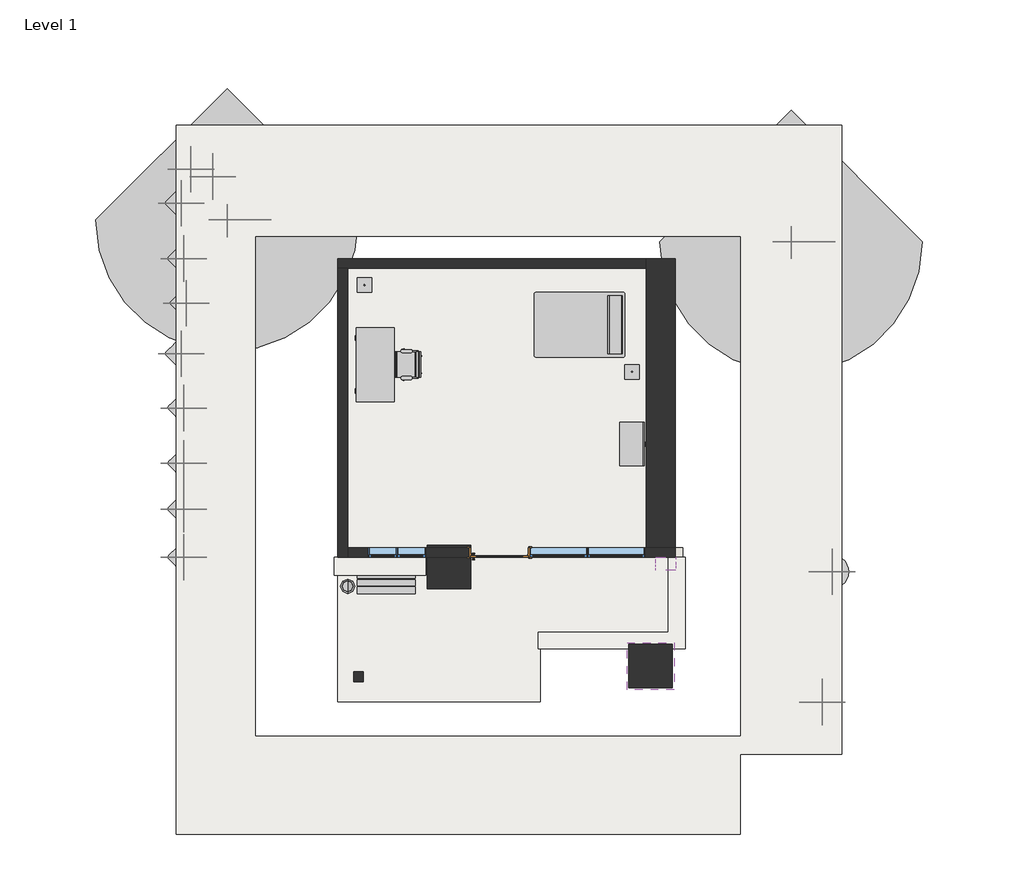
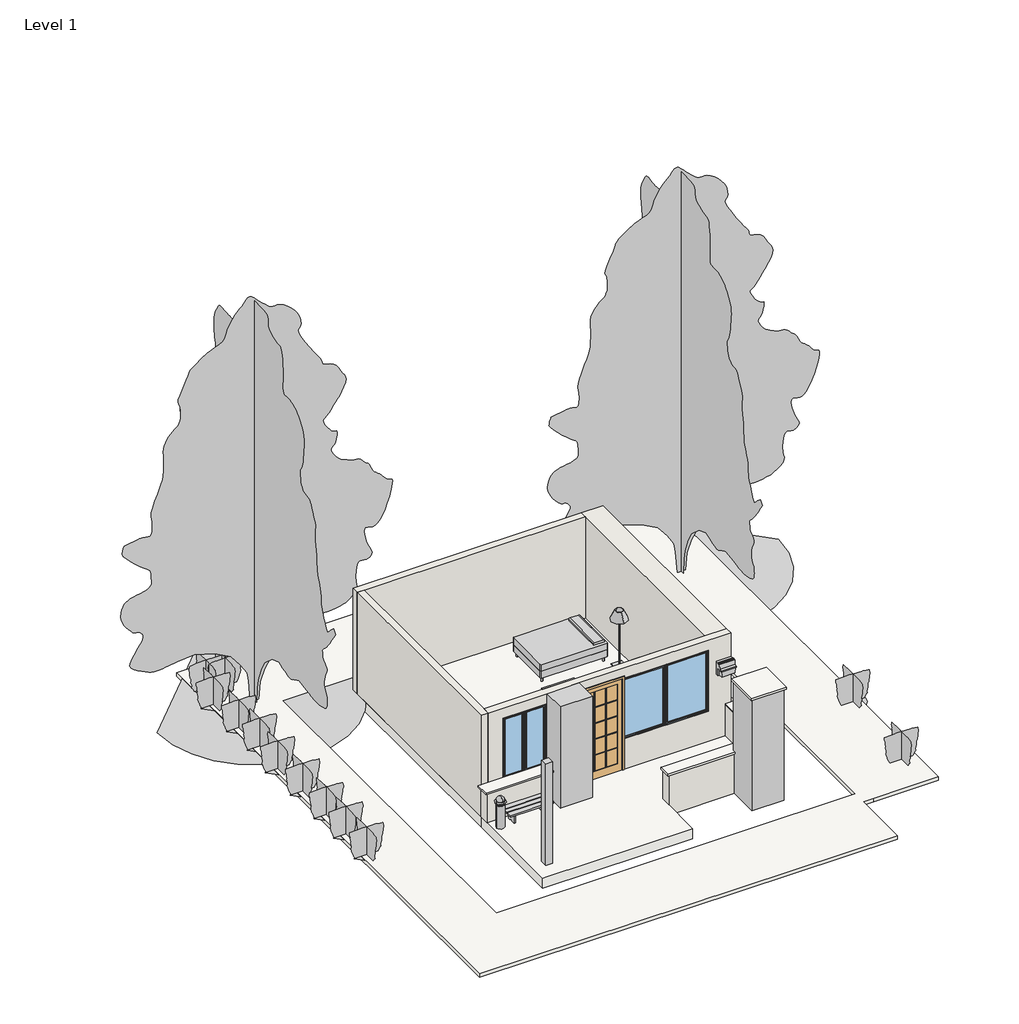
# One storey, incomplete: 14 geographic elements, 7 walls, 5 furniture elements, 5 slabs, 4 light fixtures, 4 windows, 3 columns, 1 door.
"""IFC4 building model written with IfcOpenShell, lengths in millimetres."""

from ifc_helpers import new_model, si_unit, frame, origin, origin_with_axes, place, context, project, spatial, polyline, outline, extrude, faceted_brep, transform, mapped, element, save
from components import column_81985572, door_b9d6288b, furniture_0253826f, furniture_39ce88ff, chair_task_arms_chair_task_arms_fa5a08ef, furniture_072f6425, furniture_e1dba61b, rpc_shrub_31a8b93a, rpc_tree_deciduous_lombardy_poplar_40_01077960, light_fixture_100w_120v_8564026f, bollard_light_incandescent_120v_1e792f18, wall_pack_light_exterior_120v_50d39a1a, window_a028c9d7, window_b4876e44

model = new_model("IFC4")

# Units and contexts
model_context = context("Model", 3, world=origin())
ifc_project = project(units=[si_unit("LENGTHUNIT", "METRE", prefix="MILLI")], contexts=[model_context])

# Site, building, storey
site = spatial("IfcSite", under=ifc_project)
building = spatial("IfcBuilding", under=site)
storey = spatial("IfcBuildingStorey", under=building, Name="Level 1", Elevation=0.0)

# Columns
placement = place(None, origin())
column_shape = column_81985572(model_context)
element("IfcColumn", 1, ObjectType="Rectangular Column : 18\" x 18\"", at=placement, inside=storey, context=model_context, shape_type="MappedRepresentation", body=[
    mapped(column_shape, transform((-20124.2613196, -6504.0073923, 0.0), x_axis=(1.0, 0.0, 0.0), y_axis=(0.0, 1.0, 0.0), z_axis=(0.0, 0.0, 1.0))),
])
element("IfcColumn", 2, ObjectType="Rectangular Column : 24\" x 24\" 2", at=placement, inside=storey, context=model_context, shape_type="Brep", body=[
    faceted_brep([(-17762.0613196, -3734.2582127, 3048.0), (-17762.0613196, -3734.2582127, 0.0), (-18676.4613196, -3734.2582127, 0.0), (-18676.4613196, -3734.2582127, 3048.0), (-18676.4613196, -3785.0582127, 3048.0), (-17762.0613196, -3785.0582127, 3048.0), (-17787.4613196, -3988.2582127, 2768.6), (-17787.4613196, -3988.2582127, 0.0), (-18676.4613196, -3988.2582127, 0.0), (-18676.4613196, -3988.2582127, 3048.0), (-17762.0613196, -3988.2582127, 3048.0), (-17762.0613196, -3988.2582127, 2768.6), (-17762.0613196, -4648.6582127, 0.0), (-18676.4613196, -4648.6582127, 0.0), (-18676.4613196, -4288.2957127, 0.0), (-18676.4613196, -3993.0207127, 0.0), (-17787.4613196, -3785.0582127, 0.0), (-18676.4613196, -3785.0582127, 0.0), (-17762.0613196, -3785.0582127, 2768.6), (-17762.0613196, -4648.6582127, 3048.0), (-18676.4613196, -4648.6582127, 3048.0), (-17787.4613196, -3785.0582127, 2768.6)], [[[0, 1, 2, 3]], [[0, 3, 4, 5]], [[6, 7, 8, 9, 10, 11]], [[1, 12, 13, 14, 15, 8, 7, 16, 17, 2]], [[12, 1, 0, 5, 18, 11, 10, 19]], [[13, 12, 19, 20]], [[13, 20, 9, 8, 15, 14]], [[21, 6, 11, 18]], [[21, 16, 7, 6]], [[16, 21, 18, 5, 4, 17]], [[20, 19, 10, 9]], [[3, 2, 17, 4]]]),
])
element("IfcColumn", 3, ObjectType="Rectangular Column : 24\" x 24\" 2", at=placement, inside=storey, context=model_context, shape_type="SweptSolid", body=[
    extrude(outline(polyline([(-6732.6073923, -304.8), (-6732.6073923, 3048.0), (-5818.2073923, 3048.0), (-5818.2073923, 914.4), (-5867.8582127, 914.4), (-5867.8582127, -304.8), (-6732.6073923, -304.8)])), frame((-14427.4962389, 0.0, 0.0), z_axis=(1.0, 0.0, 0.0), x_axis=(0.0, 1.0, 0.0)), (0.0, 0.0, 1.0), 914.4),
])

# Door
door_shape = door_b9d6288b(model_context)
element("IfcDoor", 4, ObjectType="Door-Interior-Single-Full Glass-Wood : 48\" x 108\"", at=placement, inside=storey, context=model_context, shape_type="MappedRepresentation", body=[
    mapped(door_shape, transform((-17152.4613196, -3889.8332127, 0.0), x_axis=(1.0, 0.0, 0.0), y_axis=(0.0, 1.0, 0.0), z_axis=(0.0, 0.0, 1.0))),
])

# Furniture
furniture_shape = furniture_0253826f(model_context)
element("IfcFurniture", 5, ObjectType="Bed-Standard : Double 54\" x 75\"", at=placement, inside=storey, context=model_context, shape_type="MappedRepresentation", body=[
    mapped(furniture_shape, transform((-15417.7662376, 1185.4303119, 0.0), x_axis=(0.0, -1.0, 0.0), y_axis=(1.0, 0.0, 0.0), z_axis=(0.0, 0.0, 1.0))),
])
furniture_2_shape = furniture_39ce88ff(model_context)
element("IfcFurniture", 6, ObjectType="Bench-Locker Room : 48\" x 18\" x 14\"", at=placement, inside=storey, context=model_context, shape_type="MappedRepresentation", body=[
    mapped(furniture_2_shape, transform((-19384.7465655, -4340.9434586, 0.0), x_axis=(1.0, 0.0, 0.0), y_axis=(0.0, 1.0, 0.0), z_axis=(0.0, 0.0, 1.0))),
])
chair_task_arms_chair_task_arms_shape = chair_task_arms_chair_task_arms_fa5a08ef(model_context)
element("IfcFurniture", 7, ObjectType="Chair-Task Arms : Chair-Task Arms", at=placement, inside=storey, context=model_context, shape_type="MappedRepresentation", body=[
    mapped(chair_task_arms_chair_task_arms_shape, transform((-19063.915418, -65.2490323, 0.0), x_axis=(0.0, 1.0000000000000002, 0.0), y_axis=(-1.0000000000000002, 0.0, 0.0), z_axis=(0.0, 0.0, 1.0))),
])
furniture_3_shape = furniture_072f6425(model_context)
element("IfcFurniture", 8, ObjectType="Desk : 60\" x 30\"", at=placement, inside=storey, context=model_context, shape_type="MappedRepresentation", body=[
    mapped(furniture_3_shape, transform((-19387.6613196, -686.2582127, 0.0), x_axis=(0.0, 1.0, 0.0), y_axis=(-1.0, 0.0, 0.0), z_axis=(0.0, 0.0, 1.0))),
])
furniture_4_shape = furniture_e1dba61b(model_context)
element("IfcFurniture", 9, ObjectType="Storage Pedestal : 20\" x 36\" x 36\"", at=placement, inside=storey, context=model_context, shape_type="MappedRepresentation", body=[
    mapped(furniture_4_shape, transform((-15292.7796957, -1420.6356987, 0.0), x_axis=(0.0, 1.0000000000000002, 0.0), y_axis=(-1.0000000000000002, 0.0, 0.0), z_axis=(0.0, 0.0, 1.0))),
])

# Geographic elements
rpc_shrub_shape = rpc_shrub_31a8b93a(model_context)
element("IfcGeographicElement", 10, ObjectType="RPC Shrub", at=placement, inside=storey, context=model_context, shape_type="MappedRepresentation", body=[
    mapped(rpc_shrub_shape, transform((-23197.6613196, 4038.1417873, 0.0), x_axis=(1.0, 0.0, 0.0), y_axis=(0.0, 1.0, 0.0), z_axis=(0.0, 0.0, 1.0))),
])
element("IfcGeographicElement", 11, ObjectType="RPC Shrub", at=placement, inside=storey, context=model_context, shape_type="MappedRepresentation", body=[
    mapped(rpc_shrub_shape, transform((-23654.8613196, 4190.5417873, 0.0), x_axis=(1.0, 0.0, 0.0), y_axis=(0.0, 1.0, 0.0), z_axis=(0.0, 0.0, 1.0))),
])
element("IfcGeographicElement", 12, ObjectType="RPC Shrub", at=placement, inside=storey, context=model_context, shape_type="MappedRepresentation", body=[
    mapped(rpc_shrub_shape, transform((-23807.2613196, 2310.9417873, 0.0), x_axis=(0.0, 1.0000000000000002, 0.0), y_axis=(-1.0000000000000002, 0.0, 0.0), z_axis=(0.0, 0.0, 1.0))),
])
element("IfcGeographicElement", 13, ObjectType="RPC Shrub", at=placement, inside=storey, context=model_context, shape_type="MappedRepresentation", body=[
    mapped(rpc_shrub_shape, transform((-23756.4613196, 1371.1417873, 0.0), x_axis=(0.0, 1.0000000000000002, 0.0), y_axis=(-1.0000000000000002, 0.0, 0.0), z_axis=(0.0, 0.0, 1.0))),
])
element("IfcGeographicElement", 14, ObjectType="RPC Shrub", at=placement, inside=storey, context=model_context, shape_type="MappedRepresentation", body=[
    mapped(rpc_shrub_shape, transform((-23858.0613196, 304.3417873, 0.0), x_axis=(0.0, 1.0000000000000002, 0.0), y_axis=(-1.0000000000000002, 0.0, 0.0), z_axis=(0.0, 0.0, 1.0))),
])
element("IfcGeographicElement", 15, ObjectType="RPC Shrub", at=placement, inside=storey, context=model_context, shape_type="MappedRepresentation", body=[
    mapped(rpc_shrub_shape, transform((-23858.0613196, 3479.3417873, 0.0), x_axis=(0.0, 1.0000000000000002, 0.0), y_axis=(-1.0000000000000002, 0.0, 0.0), z_axis=(0.0, 0.0, 1.0))),
])
element("IfcGeographicElement", 16, ObjectType="RPC Shrub", at=placement, inside=storey, context=model_context, shape_type="MappedRepresentation", body=[
    mapped(rpc_shrub_shape, transform((-23807.2613196, -838.6582127, 0.0), x_axis=(0.0, 1.0000000000000002, 0.0), y_axis=(-1.0000000000000002, 0.0, 0.0), z_axis=(0.0, 0.0, 1.0))),
])
element("IfcGeographicElement", 17, ObjectType="RPC Shrub", at=placement, inside=storey, context=model_context, shape_type="MappedRepresentation", body=[
    mapped(rpc_shrub_shape, transform((-23807.2613196, -2007.0582127, 0.0), x_axis=(0.0, 1.0000000000000002, 0.0), y_axis=(-1.0000000000000002, 0.0, 0.0), z_axis=(0.0, 0.0, 1.0))),
])
element("IfcGeographicElement", 18, ObjectType="RPC Shrub", at=placement, inside=storey, context=model_context, shape_type="MappedRepresentation", body=[
    mapped(rpc_shrub_shape, transform((-23807.2613196, -2972.2582127, 0.0), x_axis=(0.0, 1.0000000000000002, 0.0), y_axis=(-1.0000000000000002, 0.0, 0.0), z_axis=(0.0, 0.0, 1.0))),
])
element("IfcGeographicElement", 19, ObjectType="RPC Shrub", at=placement, inside=storey, context=model_context, shape_type="MappedRepresentation", body=[
    mapped(rpc_shrub_shape, transform((-23807.2613196, -3988.2582127, 0.0), x_axis=(0.0, 1.0000000000000002, 0.0), y_axis=(-1.0000000000000002, 0.0, 0.0), z_axis=(0.0, 0.0, 1.0))),
])
element("IfcGeographicElement", 20, ObjectType="RPC Shrub", at=placement, inside=storey, context=model_context, shape_type="MappedRepresentation", body=[
    mapped(rpc_shrub_shape, transform((-10142.0613196, -4293.0582127, 0.0), x_axis=(0.0, 1.0000000000000002, 0.0), y_axis=(-1.0000000000000002, 0.0, 0.0), z_axis=(0.0, 0.0, 1.0))),
])
element("IfcGeographicElement", 21, ObjectType="RPC Shrub", at=placement, inside=storey, context=model_context, shape_type="MappedRepresentation", body=[
    mapped(rpc_shrub_shape, transform((-10345.2613196, -7036.2582127, 0.0), x_axis=(0.0, 1.0000000000000002, 0.0), y_axis=(-1.0000000000000002, 0.0, 0.0), z_axis=(0.0, 0.0, 1.0))),
])
rpc_tree_deciduous_lombardy_poplar_40_shape = rpc_tree_deciduous_lombardy_poplar_40_01077960(model_context)
element("IfcGeographicElement", 22, ObjectType="RPC Tree - Deciduous : Lombardy Poplar - 40'", at=placement, inside=storey, context=model_context, shape_type="MappedRepresentation", body=[
    mapped(rpc_tree_deciduous_lombardy_poplar_40_shape, transform((-22892.8613196, 3123.7417873, 0.0), x_axis=(1.0, 0.0, 0.0), y_axis=(0.0, 1.0, 0.0), z_axis=(0.0, 0.0, 1.0))),
])
element("IfcGeographicElement", 23, ObjectType="RPC Tree - Deciduous : Lombardy Poplar - 40'", at=placement, inside=storey, context=model_context, shape_type="MappedRepresentation", body=[
    mapped(rpc_tree_deciduous_lombardy_poplar_40_shape, transform((-11005.6613196, 2666.5417873, 0.0), x_axis=(1.0, 0.0, 0.0), y_axis=(0.0, 1.0, 0.0), z_axis=(0.0, 0.0, 1.0))),
])

# Light fixtures
light_fixture_100w_120v_shape = light_fixture_100w_120v_8564026f(model_context)
element("IfcLightFixture", 24, ObjectType="100W - 120V", at=placement, inside=storey, context=model_context, shape_type="MappedRepresentation", body=[
    mapped(light_fixture_100w_120v_shape, transform((-14358.4613196, -76.6582127, 0.0), x_axis=(1.0, 0.0, 0.0), y_axis=(0.0, 1.0, 0.0), z_axis=(0.0, 0.0, 1.0))),
])
element("IfcLightFixture", 25, ObjectType="100W - 120V", at=placement, inside=storey, context=model_context, shape_type="MappedRepresentation", body=[
    mapped(light_fixture_100w_120v_shape, transform((-19997.2613196, 1752.1417873, 0.0), x_axis=(1.0, 0.0, 0.0), y_axis=(0.0, 1.0, 0.0), z_axis=(0.0, 0.0, 1.0))),
])
bollard_light_incandescent_120v_shape = bollard_light_incandescent_120v_1e792f18(model_context)
element("IfcLightFixture", 26, ObjectType="Bollard Light : Incandescent - 120V", at=placement, inside=storey, context=model_context, shape_type="MappedRepresentation", body=[
    mapped(bollard_light_incandescent_120v_shape, transform((-20238.5613196, -4483.5582127, 0.0), x_axis=(1.0, 0.0, 0.0), y_axis=(0.0, 1.0, 0.0), z_axis=(0.0, 0.0, 1.0))),
])
wall_pack_light_exterior_120v_shape = wall_pack_light_exterior_120v_50d39a1a(model_context)
element("IfcLightFixture", 27, ObjectType="Wall Pack Light - Exterior : 120V", at=placement, inside=storey, context=model_context, shape_type="MappedRepresentation", body=[
    mapped(wall_pack_light_exterior_120v_shape, transform((-13525.4972631, -3886.6582127, -410.5667895), x_axis=(-1.0, 0.0, 0.0), y_axis=(0.0, -1.0, 0.0), z_axis=(0.0, 0.0, 1.0))),
])

# Slabs
element("IfcSlab", 28, ObjectType="Generic - 12\" 2", at=placement, inside=storey, context=model_context, shape_type="SweptSolid", body=[
    extrude(outline(polyline([(-16339.6613196, -5563.0582127), (-16288.8613196, -5563.0582127), (-13596.4613196, -5563.0582127), (-13596.4613196, -3988.2582127), (-13240.8613196, -3988.2582127), (-13240.8613196, -5918.6582127), (-16339.6613196, -5918.6582127), (-16339.6613196, -5563.0582127)])), frame((0.0, 0.0, 914.4), z_axis=(0.0, 0.0, 1.0), x_axis=(1.0, 0.0, 0.0)), (0.0, 0.0, 1.0), 50.8),
])
element("IfcSlab", 29, ObjectType="Generic - 12\" 2", at=placement, inside=storey, context=model_context, shape_type="SweptSolid", body=[
    extrude(outline(polyline([(-13471.6313793, -5783.9576353), (-13471.6313793, -6774.5576353), (-14462.2313793, -6774.5576353), (-14462.2313793, -5783.9576353), (-13471.6313793, -5783.9576353)])), frame((0.0, 0.0, 3048.0), z_axis=(0.0, 0.0, 1.0), x_axis=(1.0, 0.0, 0.0)), (0.0, 0.0, 1.0), 50.8),
])
element("IfcSlab", 30, ObjectType="Generic - 12\" 2", at=placement, inside=storey, context=model_context, shape_type="SweptSolid", body=[
    extrude(outline(polyline([(-20632.2613196, -3988.2582127), (-18701.8613196, -3988.2582127), (-18701.8613196, -4369.2582127), (-20632.2613196, -4369.2582127), (-20632.2613196, -3988.2582127)])), frame((0.0, 0.0, 914.4), z_axis=(0.0, 0.0, 1.0), x_axis=(1.0, 0.0, 0.0)), (0.0, 0.0, 1.0), 50.8),
])
element("IfcSlab", 31, ObjectType="Generic - 12\" 4", at=placement, inside=storey, context=model_context, shape_type="SweptSolid", body=[
    extrude(outline(polyline([(-20556.0613196, -3988.2582127), (-20556.0613196, 2310.9417873), (-13444.0613196, 2310.9417873), (-13444.0613196, -5715.4582127), (-16288.8613196, -5715.4582127), (-16288.8613196, -7036.2582127), (-20556.0613196, -7036.2582127), (-20556.0613196, -3988.2582127)])), frame((0.0, 0.0, -304.8), z_axis=(0.0, 0.0, 1.0), x_axis=(1.0, 0.0, 0.0)), (0.0, 0.0, 1.0), 304.8),
])
element("IfcSlab", 32, ObjectType="LW Concrete on Metal Deck", at=placement, inside=storey, context=model_context, shape_type="SweptSolid", body=[
    extrude(outline(polyline([(-9941.1630617, 5115.9853444), (-9941.1630617, -8142.8146556), (-11769.9630617, -8142.8146556), (-12074.7630617, -8142.8146556), (-12074.7630617, -9819.2146556), (-23961.9630617, -9819.2146556), (-23961.9630617, 5115.9853444), (-9941.1630617, 5115.9853444)]), holes=[polyline([(-12074.7630617, 2310.9417873), (-12074.7630617, 2768.1417873), (-22285.5630617, 2768.1417873), (-22285.5630617, -7747.4582127), (-12074.7630617, -7747.4582127), (-12074.7630617, 2310.9417873)])]), frame((0.0, 0.0, -104.775), z_axis=(0.0, 0.0, 1.0), x_axis=(1.0, 0.0, 0.0)), (0.0, 0.0, 1.0), 104.775),
])

# Walls
element("IfcWall", 33, ObjectType="Generic - 12\"", at=placement, inside=storey, context=model_context, shape_type="Brep", body=[
    faceted_brep([(-16288.8613196, -5867.8582127, -304.8), (-14427.4962389, -5867.8582127, -304.8), (-13513.0962389, -5867.8582127, -304.8), (-13291.6613196, -5867.8582127, -304.8), (-13291.6613196, -5867.8582127, 914.4), (-13513.0962389, -5867.8582127, 914.4), (-14427.4962389, -5867.8582127, 914.4), (-16288.8613196, -5867.8582127, 914.4), (-16288.8613196, -5563.0582127, -304.8), (-16288.8613196, -5563.0582127, 914.4), (-13596.4613196, -5563.0582127, 914.4), (-13291.6613196, -5563.0582127, 914.4), (-13291.6613196, -5563.0582127, -304.8), (-13596.4613196, -5563.0582127, -304.8)], [[[0, 1, 2, 3, 4, 5, 6, 7]], [[8, 9, 10, 11, 12, 13]], [[3, 2, 1, 0, 8, 13, 12]], [[7, 6, 5, 4, 11, 10, 9]], [[0, 7, 9, 8]], [[4, 3, 12, 11]]]),
])
element("IfcWall", 34, ObjectType="Generic - 12\"", at=placement, inside=storey, context=model_context, shape_type="Brep", body=[
    faceted_brep([(-13291.6613196, -5563.0582127, -304.8), (-13291.6613196, -3988.2582127, -304.8), (-13291.6613196, -3988.2582127, 0.0), (-13291.6613196, -3988.2582127, 914.4), (-13291.6613196, -5563.0582127, 914.4), (-13596.4613196, -5563.0582127, -304.8), (-13596.4613196, -5563.0582127, 914.4), (-13596.4613196, -3988.2582127, 914.4), (-13596.4613196, -3988.2582127, -304.8), (-13444.0613196, -3988.2582127, 914.4)], [[[0, 1, 2, 3, 4]], [[5, 6, 7, 8]], [[1, 0, 5, 8]], [[4, 3, 9, 7, 6]], [[0, 4, 6, 5]], [[3, 2, 1, 8, 7, 9]]]),
])
element("IfcWall", 35, ObjectType="Generic - 12\" Masonry", at=placement, inside=storey, context=model_context, shape_type="SweptSolid", body=[
    extrude(outline(polyline([(-18676.4613196, -4288.2957127), (-20556.0613196, -4288.2957127), (-20556.0613196, -3993.0207127), (-18676.4613196, -3993.0207127), (-18676.4613196, -4288.2957127)])), origin_with_axes(), (0.0, 0.0, 1.0), 914.4),
])
element("IfcWall", 36, ObjectType="Generic - 8\"", at=placement, inside=storey, context=model_context, shape_type="Brep", body=[
    faceted_brep([(-20556.0613196, 2107.7417873, 0.0), (-20352.8613196, 2107.7417873, 0.0), (-14053.6613196, 2107.7417873, 0.0), (-14053.6613196, 2107.7417873, 3048.0), (-20352.8613196, 2107.7417873, 3048.0), (-20556.0613196, 2107.7417873, 3048.0), (-20556.0613196, 2310.9417873, 0.0), (-20556.0613196, 2310.9417873, 3048.0), (-14053.6613196, 2310.9417873, 3048.0), (-14053.6613196, 2310.9417873, 0.0)], [[[0, 1, 2, 3, 4, 5]], [[6, 7, 8, 9]], [[2, 1, 0, 6, 9]], [[0, 5, 7, 6]], [[3, 2, 9, 8]], [[5, 4, 3, 8, 7]]]),
])
element("IfcWall", 37, ObjectType="Generic - 8\"", at=placement, inside=storey, context=model_context, shape_type="Brep", body=[
    faceted_brep([(-20352.8613196, -3988.2582127, 0.0), (-20352.8613196, -3785.0582127, 0.0), (-20352.8613196, 2107.7417873, 0.0), (-20352.8613196, 2107.7417873, 3048.0), (-20352.8613196, -3785.0582127, 3048.0), (-20352.8613196, -3988.2582127, 3048.0), (-20556.0613196, -3988.2582127, 0.0), (-20556.0613196, -3988.2582127, 3048.0), (-20556.0613196, 2107.7417873, 3048.0), (-20556.0613196, 2107.7417873, 0.0)], [[[0, 1, 2, 3, 4, 5]], [[6, 7, 8, 9]], [[2, 1, 0, 6, 9]], [[0, 5, 7, 6]], [[3, 2, 9, 8]], [[5, 4, 3, 8, 7]]]),
])
element("IfcWall", 38, ObjectType="Generic - 8\"", at=placement, inside=storey, context=model_context, shape_type="Brep", body=[
    faceted_brep([(-20352.8613196, -3785.0582127, 0.0), (-20352.8613196, -3785.0582127, 3048.0), (-18676.4613196, -3785.0582127, 3048.0), (-17762.0613196, -3785.0582127, 3048.0), (-14053.6613196, -3785.0582127, 3048.0), (-13444.0613196, -3785.0582127, 3048.0), (-13444.0613196, -3785.0582127, 914.4), (-13291.6613196, -3785.0582127, 914.4), (-13291.6613196, -3785.0582127, 0.0), (-13444.0613196, -3785.0582127, 0.0), (-14053.6613196, -3785.0582127, 0.0), (-16517.4613196, -3785.0582127, 0.0), (-16517.4613196, -3785.0582127, 911.4953017), (-14079.0613196, -3785.0582127, 911.4953017), (-14079.0613196, -3785.0582127, 2740.2953017), (-16517.4613196, -3785.0582127, 2740.2953017), (-16517.4613196, -3785.0582127, 2768.6), (-17762.0613196, -3785.0582127, 2768.6), (-17787.4613196, -3785.0582127, 2768.6), (-17787.4613196, -3785.0582127, 0.0), (-18676.4613196, -3785.0582127, 0.0), (-19921.0613196, -3785.0582127, 2740.2953017), (-19921.0613196, -3785.0582127, 911.4953017), (-18701.8613196, -3785.0582127, 911.4953017), (-18701.8613196, -3785.0582127, 2740.2953017), (-20352.8613196, -3988.2582127, 3048.0), (-20352.8613196, -3988.2582127, 0.0), (-18676.4613196, -3988.2582127, 0.0), (-17787.4613196, -3988.2582127, 0.0), (-17787.4613196, -3988.2582127, 2768.6), (-17762.0613196, -3988.2582127, 2768.6), (-16517.4613196, -3988.2582127, 2768.6), (-16517.4613196, -3988.2582127, 2740.2953017), (-14079.0613196, -3988.2582127, 2740.2953017), (-14079.0613196, -3988.2582127, 911.4953017), (-16517.4613196, -3988.2582127, 911.4953017), (-16517.4613196, -3988.2582127, 0.0), (-13291.6613196, -3988.2582127, 0.0), (-13291.6613196, -3988.2582127, 914.4), (-13444.0613196, -3988.2582127, 914.4), (-13444.0613196, -3988.2582127, 3048.0), (-17762.0613196, -3988.2582127, 3048.0), (-18676.4613196, -3988.2582127, 3048.0), (-19921.0613196, -3988.2582127, 911.4953017), (-19921.0613196, -3988.2582127, 2740.2953017), (-18701.8613196, -3988.2582127, 2740.2953017), (-18701.8613196, -3988.2582127, 911.4953017)], [[[0, 1, 2, 3, 4, 5, 6, 7, 8, 9, 10, 11, 12, 13, 14, 15, 16, 17, 18, 19, 20], [21, 22, 23, 24]], [[25, 26, 27, 28, 29, 30, 31, 32, 33, 34, 35, 36, 37, 38, 39, 40, 41, 42], [43, 44, 45, 46]], [[8, 37, 36, 11, 10, 9]], [[26, 0, 20, 19, 28, 27]], [[1, 0, 26, 25]], [[11, 36, 35, 12]], [[31, 16, 15, 32]], [[18, 17, 16, 31, 30, 29]], [[19, 18, 29, 28]], [[22, 43, 46, 23]], [[43, 22, 21, 44]], [[44, 21, 24, 45]], [[45, 24, 23, 46]], [[12, 35, 34, 13]], [[14, 33, 32, 15]], [[33, 14, 13, 34]], [[39, 38, 7, 6]], [[37, 8, 7, 38]], [[6, 5, 40, 39]], [[5, 4, 3, 2, 1, 25, 42, 41, 40]]]),
])
element("IfcWall", 39, ObjectType="Generic - 8\" 2", at=placement, inside=storey, context=model_context, shape_type="Brep", body=[
    faceted_brep([(-14053.6613196, 2310.9417873, 0.0), (-14053.6613196, 2107.7417873, 0.0), (-14053.6613196, -3785.0582127, 0.0), (-14053.6613196, -3785.0582127, 3048.0), (-14053.6613196, 2107.7417873, 3048.0), (-14053.6613196, 2310.9417873, 3048.0), (-13444.0613196, 2310.9417873, 0.0), (-13444.0613196, 2310.9417873, 3048.0), (-13444.0613196, -3785.0582127, 3048.0), (-13444.0613196, -3785.0582127, 914.4), (-13444.0613196, -3785.0582127, 0.0)], [[[0, 1, 2, 3, 4, 5]], [[6, 7, 8, 9, 10]], [[2, 1, 0, 6, 10]], [[0, 5, 7, 6]], [[5, 4, 3, 8, 7]], [[3, 2, 10, 9, 8]]]),
])

# Windows
window_shape = window_a028c9d7(model_context)
element("IfcWindow", 40, ObjectType="Fixed : 24\" x 72\"", at=placement, inside=storey, context=model_context, shape_type="MappedRepresentation", body=[
    mapped(window_shape, transform((-19578.1613196, -3886.6582127, 606.6953017), x_axis=(1.0, 0.0, 0.0), y_axis=(0.0, 1.0, 0.0), z_axis=(0.0, 0.0, 1.0))),
])
element("IfcWindow", 41, ObjectType="Fixed : 24\" x 72\"", at=placement, inside=storey, context=model_context, shape_type="MappedRepresentation", body=[
    mapped(window_shape, transform((-18968.5613196, -3886.6582127, 606.6953017), x_axis=(1.0, 0.0, 0.0), y_axis=(0.0, 1.0, 0.0), z_axis=(0.0, 0.0, 1.0))),
])
window_2_shape = window_b4876e44(model_context)
element("IfcWindow", 42, ObjectType="Fixed : 48\" x 72\"", at=placement, inside=storey, context=model_context, shape_type="MappedRepresentation", body=[
    mapped(window_2_shape, transform((-15869.7613196, -3886.6582127, 606.6953017), x_axis=(1.0, 0.0, 0.0), y_axis=(0.0, 1.0, 0.0), z_axis=(0.0, 0.0, 1.0))),
])
element("IfcWindow", 43, ObjectType="Fixed : 48\" x 72\"", at=placement, inside=storey, context=model_context, shape_type="MappedRepresentation", body=[
    mapped(window_2_shape, transform((-14650.5613196, -3886.6582127, 606.6953017), x_axis=(1.0, 0.0, 0.0), y_axis=(0.0, 1.0, 0.0), z_axis=(0.0, 0.0, 1.0))),
])

save(model, "model.ifc")

# Revit data of these elements
# Type "Rectangular Column : 18\" x 18\""
#   Assembly Code = "B1010200"
#   Depth = 0' - 8"
#   Offset Base = 0' - 0"
#   Offset Top = 0' - 0"
#   Width = 0' - 8"
#   Material = Stainless Steel
# Type "Rectangular Column : 24\" x 24\" 2"
#   Assembly Code = "B1010200"
#   Depth = 3' - 0"
#   Offset Base = 0' - 0"
#   Offset Top = 0' - 0"
#   Width = 3' - 0"
#   Material = Iron, Ductile
# Type "Door-Interior-Single-Full Glass-Wood : 48\" x 108\""
#   Type Mark = "10"
#   Assembly Code = "C1020300"
#   Analytic Construction = "Wood frame with single clear glass"
#   Top Rail = 0' - 4 11/16"
#   Thickness = 0' - 1 3/8"
#   Thermal Resistance (R) = 1.0102 (h·ft²·°F)/BTU
#   Swing Angle [instance default] = 90.00°
#   Stiles = 0' - 4 3/4"
#   Rough Width = 4' - 2"
#   Rough Height = 9' - 1"
#   Height = 9' - 0"
#   Width = 4' - 0"
#   Heat Transfer Coefficient (U) = 0.9900 BTU/(h·ft²·°F)
#   Bottom Rail = 0' - 9 1/8"
#   Show Grill [instance default] = yes
#   Trim Material = Cherry
#   Panel Material = Brick, Common
#   Frame Material = Cherry
#   Door Handle Material = Aluminum
#   Visual Light Transmittance = 0
#   Solar Heat Gain Coefficient = 0
#   Wall Closure = (empty or 0)
#   Function = (empty or 0)
# Type "Bed-Standard : Double 54\" x 75\""
#   Assembly Code = "E2020200"
#   Length = 6' - 3"
#   Width = 4' - 6"
#   Leg Material = Steel, Chrome Plated
#   Mattress Material = Linen, White
#   Default Elevation = 0
# Type "Bench-Locker Room : 48\" x 18\" x 14\""
#   Assembly Code = "E2020200"
#   Depth = 1' - 6"
#   Height = 1' - 2"
#   Width = 4' - 0"
#   Bench Material = Cherry
#   Default Elevation = 0
# Type "Chair-Task Arms : Chair-Task Arms"
#   Assembly Code = "E2020200"
#   Base Material = Plastic, Opaque Black
#   Caster Material = Plastic, Opaque Black
#   Seat/Back Material = Textile - Slate Blue
#   Default Elevation = 0
# Type "Desk : 60\" x 30\""
#   Assembly Code = "E2020200"
#   Depth = 2' - 6"
#   Height = 2' - 6"
#   Leg Height = 0' - 6"
#   Width = 5' - 0"
#   Body Material = Laminate, Ivory, Matte
#   Handle/Leg Material = Steel, Chrome Plated
#   Top Material = Cherry
#   Default Elevation = 0
# Type "Storage Pedestal : 20\" x 36\" x 36\""
#   Assembly Code = "E2020"
#   Depth = 1' - 8"
#   Height = 3' - 0"
#   Width = 3' - 0"
#   Cabinet Material = Steel, Paint Finish, Ivory, Glossy
#   Handles Material = Steel, Chrome Plated
#   Default Elevation = 0
# Type "RPC Shrub"
#   Type Comments = "Boxwood"
#   built-in parameter 1005198 = "{2, 15},{39, RPC-16-G0M3-8AG0-UBW3-U000-ST1L-LVER-AU},{1, 0},{1, 0},{2, 13},{1, 8},{5, Color},{1, 0},{1, 0},{3, 0.8},{3, 0.8},{3, 0.8},{1, 8},{7, BBoxMin},{1, 0},{1, 0},{1, 0},{1, 0},{1, 0},{1, 8},{7, BBoxMax},{1, 0},{1, 0},{1, 0},{1, 0},{1, 0},{2, 11},{9, RPCTypeId},{1, 0},{1, 0},{39, RPC-16-G0M3-8AG0-UBW3-U000-ST1L-LVER-AU},{1, 6},{14, RPCPlantHeight},{1, 0},{1, 0},{4, 2.75},{2, 11},{7, keyword},{1, 0},{1, 0},{35, :RPCs:Shrubs & Grasses:Geometry:RPC},{2, 11},{8, category},{1, 0},{1, 0},{16, Shrubs & Grasses},{2, 11},{12, LocalizedUID},{1, 0},{1, 0},{7, Boxwood},{2, 14},{6, Height},{1, 0},{1, 0},{4, 2.75},{1, 2},{16, Cast Reflections},{1, 0},{1, 0},{1, 0},{1, 2},{12, Cast Shadows},{1, 0},{1, 0},{1, 1},{1, 2},{9, Lock View},{1, 0},{1, 0},{1, 0},{1, 4},{5, ViewC},{1, 0},{1, 0},{1, 0},{21, assetlibrary_base.fbx},{1, 5},"
#   built-in parameter 1005195 = "RPC-16-G0M3-8AG0-UBW3-U000-ST1L-LVER-AU"
#   Assembly Code = "G2050500"
#   Height = 2' - 9"
#   Default Elevation = 0
# Type "RPC Tree - Deciduous : Lombardy Poplar - 40'"
#   built-in parameter 1005198 = "{2, 15},{39, RPC-16-FVA4-CP7X-CFP7-S000-ST1L-LVER-AU},{1, 0},{1, 0},{2, 13},{1, 8},{5, Color},{1, 0},{1, 0},{3, 0.8},{3, 0.8},{3, 0.8},{1, 8},{7, BBoxMin},{1, 0},{1, 0},{1, 0},{1, 0},{1, 0},{1, 8},{7, BBoxMax},{1, 0},{1, 0},{1, 0},{1, 0},{1, 0},{2, 11},{9, RPCTypeId},{1, 0},{1, 0},{39, RPC-16-FVA4-CP7X-CFP7-S000-ST1L-LVER-AU},{1, 6},{14, RPCPlantHeight},{1, 0},{1, 0},{2, 40},{2, 11},{7, keyword},{1, 0},{1, 0},{34, :RPCs:Trees [General]:Geometry:RPC},{2, 11},{8, category},{1, 0},{1, 0},{15, Trees [General]},{2, 11},{12, LocalizedUID},{1, 0},{1, 0},{15, Lombardy Poplar},{2, 14},{6, Height},{1, 0},{1, 0},{2, 40},{1, 2},{16, Cast Reflections},{1, 0},{1, 0},{1, 0},{1, 2},{12, Cast Shadows},{1, 0},{1, 0},{1, 1},{1, 2},{9, Lock View},{1, 0},{1, 0},{1, 0},{1, 4},{5, ViewC},{1, 0},{1, 0},{1, 0},{21, assetlibrary_base.fbx},{1, 5},"
#   built-in parameter 1005195 = "RPC-16-FVA4-CP7X-CFP7-S000-ST1L-LVER-AU"
#   Type Comments = "Lombardy Poplar"
#   Assembly Code = "G2050500"
#   Height = 40' - 0"
#   Default Elevation = 0
# Type "100W - 120V"
#   Assembly Code = "D5020220"
#   Lamp = "A-19"
#   Wattage Comments = "100"
#   Wattage = 100 W
#   built-in parameter 1150110 = 1 (stored number, unit not read)
#   built-in parameter 1114217 = 1 (stored number, unit not read)
#   built-in parameter 1150109 = 1 (stored number, unit not read)
#   built-in parameter 1150113 = 1 (stored number, unit not read)
#   built-in parameter 1150115 = 1 (stored number, unit not read)
#   built-in parameter 1150105 = 139.261 (stored number, unit not read)
#   Light Source Symbol Size = 2' - 0"
#   built-in parameter 1150112 = 1 (stored number, unit not read)
#   built-in parameter 1150114 = 1 (stored number, unit not read)
#   built-in parameter 1150107 = 2800 (stored number, unit not read)
#   built-in parameter 1150106 = 1.39261 (stored number, unit not read)
#   built-in parameter 1150104 = 1.6258 (stored number, unit not read)
#   Ballast Voltage = 120 V
#   built-in parameter 1114218 = 1 (stored number, unit not read)
#   built-in parameter 1150133 = 10 (stored number, unit not read)
#   Lumens = 1750 lm
#   Apparent Load = 100 VA
#   built-in parameter 1150134 = 4
#   built-in parameter 1150137 = 1
#   Color Filter = 16777215
#   Ballast Number of Poles = 1
#   Shade = Glass, Frosted
#   Stand = Steel, Chrome Plated
#   Dimming Lamp Color Temperature Shift = (empty or 0)
#   Default Elevation = 0
# Type "Bollard Light : Incandescent - 120V"
#   Lamp = "A-19"
#   Wattage = 100 W
#   built-in parameter 1150110 = 1 (stored number, unit not read)
#   built-in parameter 1114217 = 1 (stored number, unit not read)
#   built-in parameter 1150109 = 1 (stored number, unit not read)
#   built-in parameter 1150113 = 1 (stored number, unit not read)
#   Lumens = 1690 lm
#   built-in parameter 1150115 = 1 (stored number, unit not read)
#   built-in parameter 1150105 = 134.486 (stored number, unit not read)
#   Light Source Symbol Size = 2' - 0"
#   built-in parameter 1150112 = 1 (stored number, unit not read)
#   built-in parameter 1150114 = 1 (stored number, unit not read)
#   built-in parameter 1150107 = 2800 (stored number, unit not read)
#   built-in parameter 1150106 = 1.34486 (stored number, unit not read)
#   built-in parameter 1150104 = 1.57006 (stored number, unit not read)
#   Ballast Voltage = 120 V
#   built-in parameter 1114218 = 1 (stored number, unit not read)
#   built-in parameter 1150133 = 10 (stored number, unit not read)
#   Apparent Load = 100 VA
#   built-in parameter 1150134 = 4
#   built-in parameter 1150137 = 1
#   Color Filter = 16777215
#   Ballast Number of Poles = 1
#   Load Classification = Lighting - Exterior
#   Dimming Lamp Color Temperature Shift = (empty or 0)
#   Default Elevation = 0
# Type "Wall Pack Light - Exterior : 120V"
#   Assembly Code = "D5020230"
#   Wattage = 70 W
#   built-in parameter 1150110 = 1 (stored number, unit not read)
#   built-in parameter 1114217 = 1 (stored number, unit not read)
#   built-in parameter 1150109 = 1 (stored number, unit not read)
#   built-in parameter 1150113 = 1 (stored number, unit not read)
#   built-in parameter 1150115 = 1 (stored number, unit not read)
#   built-in parameter 1150105 = 437.668 (stored number, unit not read)
#   Light Source Symbol Size = 2' - 0"
#   built-in parameter 1150112 = 1 (stored number, unit not read)
#   built-in parameter 1150114 = 1 (stored number, unit not read)
#   built-in parameter 1150107 = 4000 (stored number, unit not read)
#   built-in parameter 1150106 = 4.37668 (stored number, unit not read)
#   built-in parameter 1150104 = 7.29939 (stored number, unit not read)
#   Ballast Voltage = 120 V
#   built-in parameter 1114218 = 1 (stored number, unit not read)
#   built-in parameter 1150133 = 10 (stored number, unit not read)
#   Lumens = 5499.9 lm
#   Mounting Height = 9' - 0"
#   Apparent Load = 70 VA
#   built-in parameter 1150134 = 12
#   built-in parameter 1150137 = 1
#   Color Filter = 16777215
#   Ballast Number of Poles = 1
#   Wall Mount Material = Metal - Paint Finish - Dark Grey, Matte
#   Shade Material = Glass
#   Load Classification = Lighting - Exterior
#   Dimming Lamp Color Temperature Shift = (empty or 0)
#   Default Elevation = 0
# Type "Generic - 12\" 2"
#   Assembly Code = "B1010"
#   Function = 0
#   Layers, outside or top first: 0' - 2" "Vinyl Composition Tile" (function 1)
# Type "Generic - 12\" 4"
#   Assembly Code = "B1010"
#   Function = 0
#   Layers, outside or top first: 1' - 0" "Roofing, EPDM Membrane" (function 1)
# Type "LW Concrete on Metal Deck"
#   Assembly Code = "B1010"
#   Function = 0
#   Layers, outside or top first: 0' - 4" "Concrete, Lightweight" (function 1); 0' - 0 1/8" "Metal Deck" (function 1)
# Type "Generic - 12\""
#   Assembly Code = "B2010"
#   Layers, outside or top first: 1' - 0" no material (function 1)
# Type "Generic - 12\" Masonry"
#   Assembly Code = "B2010"
#   Layers, outside or top first: 0' - 11 5/8" "Concrete Masonry Units" (function 1)
# Type "Generic - 8\""
#   Assembly Code = "B2010"
#   Layers, outside or top first: 0' - 8" "Brick, Soldier Course" (function 1)
# Type "Generic - 8\" 2"
#   Assembly Code = "B2010"
#   Layers, outside or top first: 2' - 0" "Brick, Soldier Course" (function 1)
# Type "Fixed : 24\" x 72\""
#   Type Mark = "14"
#   Construction Type Id = "GSP4R"
#   Assembly Code = "B2020100"
#   Analytic Construction = "1/8 in Pilkington single glazing"
#   Visual Light Transmittance = 0.9
#   Solar Heat Gain Coefficient = 0.78
#   Heat Transfer Coefficient (U) = 0.6496 BTU/(h·ft²·°F)
#   Height = 6' - 0"
#   Default Sill Height = 1' - 0"
#   Width = 2' - 0"
#   Window Inset = 0' - 6"
#   Define Thermal Properties by = 1
#   Glass Pane Material = Glass
#   Sash Material = Structure, Steel Bar Joist Layer
#   Wall Closure = (empty or 0)
# Type "Fixed : 48\" x 72\""
#   Type Mark = "13"
#   Construction Type Id = "GSP4R"
#   Assembly Code = "B2020100"
#   Analytic Construction = "1/8 in Pilkington single glazing"
#   Visual Light Transmittance = 0.9
#   Solar Heat Gain Coefficient = 0.78
#   Heat Transfer Coefficient (U) = 0.6496 BTU/(h·ft²·°F)
#   Height = 6' - 0"
#   Default Sill Height = 1' - 0"
#   Width = 4' - 0"
#   Window Inset = 0' - 6"
#   Define Thermal Properties by = 1
#   Glass Pane Material = Glass
#   Sash Material = Structure, Steel Bar Joist Layer
#   Wall Closure = (empty or 0)
# Element 1 (IfcColumn, "Rectangular Column : 18\" x 18\"")
#   Phase Created = New Construction
#   Materials on its faces: "Stainless Steel"
# Element 2 (IfcColumn, "Rectangular Column : 24\" x 24\" 2")
#   Phase Created = New Construction
#   Materials on its faces: "Iron, Ductile", "Oak Flooring", "Roofing, EPDM Membrane"
# Element 3 (IfcColumn, "Rectangular Column : 24\" x 24\" 2")
#   Phase Created = New Construction
#   Materials on its faces: "Iron, Ductile"
# Element 4 (IfcDoor, "Door-Interior-Single-Full Glass-Wood : 48\" x 108\"")
#   Swing Angle = 90.00°
#   Show Grill = yes
#   Phase Created = New Construction
#   Materials on its faces: "Brick, Common", "Cherry", "Aluminum", "Glass"
# Element 5 (IfcFurniture, "Bed-Standard : Double 54\" x 75\"")
#   Phase Created = New Construction
#   Materials on its faces: "Linen, White", "Steel, Chrome Plated"
# Element 6 (IfcFurniture, "Bench-Locker Room : 48\" x 18\" x 14\"")
#   Phase Created = New Construction
#   Materials on its faces: "Cherry"
# Element 7 (IfcFurniture, "Chair-Task Arms : Chair-Task Arms")
#   Phase Created = New Construction
#   Materials on its faces: "Plastic, Opaque Black", "Textile - Slate Blue"
# Element 8 (IfcFurniture, "Desk : 60\" x 30\"")
#   Phase Created = New Construction
#   Materials on its faces: "Steel, Chrome Plated", "Laminate, Ivory, Matte", "Cherry"
# Element 9 (IfcFurniture, "Storage Pedestal : 20\" x 36\" x 36\"")
#   Phase Created = New Construction
#   Materials on its faces: "Steel, Paint Finish, Ivory, Glossy", "Steel, Chrome Plated"
# Elements 10, 11, 12, 13, 14, 15, 16, 17, 18, 19, 20, 21 (IfcGeographicElement, "RPC Shrub")
#   Phase Created = New Construction
# Elements 22, 23 (IfcGeographicElement, "RPC Tree - Deciduous : Lombardy Poplar - 40'")
#   Phase Created = New Construction
# Element 24 (IfcLightFixture, "100W - 120V")
#   Mark = "1"
#   Phase Created = New Construction
#   Materials on its faces: "Steel, Chrome Plated", "Glass, Frosted"
# Element 25 (IfcLightFixture, "100W - 120V")
#   Mark = "2"
#   Phase Created = New Construction
#   Materials on its faces: "Steel, Chrome Plated", "Glass, Frosted"
# Element 26 (IfcLightFixture, "Bollard Light : Incandescent - 120V")
#   Mark = "5"
#   Phase Created = New Construction
#   Materials on its faces: "Steel, Polished", "Glass", "Concrete, Precast"
# Element 27 (IfcLightFixture, "Wall Pack Light - Exterior : 120V")
#   Mark = "3"
#   Phase Created = New Construction
#   Materials on its faces: "Metal - Paint Finish - Dark Grey, Matte", "Glass"
# Elements 28, 30 (IfcSlab, "Generic - 12\" 2")
#   built-in parameter 1001955 = 3.14159 (stored number, unit not read)
#   Height Offset From Level = 3' - 2"
#   Phase Created = New Construction
#   Materials on its faces: "Vinyl Composition Tile"
# Element 29 (IfcSlab, "Generic - 12\" 2")
#   Height Offset From Level = 10' - 2"
#   Phase Created = New Construction
#   Materials on its faces: "Vinyl Composition Tile"
# Element 31 (IfcSlab, "Generic - 12\" 4")
#   built-in parameter 1001955 = -1.5708 (stored number, unit not read)
#   Height Offset From Level = 0' - 0"
#   Phase Created = New Construction
#   Materials on its faces: "Roofing, EPDM Membrane"
# Element 32 (IfcSlab, "LW Concrete on Metal Deck")
#   Height Offset From Level = 0' - 0"
#   Phase Created = New Construction
#   Materials on its faces: "Metal Deck", "Concrete, Lightweight"
# Element 33 (IfcWall, "Generic - 12\"")
#   built-in parameter 1001111 = -1' - 0"
#   Top Offset = 0' - 0"
#   Base Offset = -1' - 0"
#   Unconnected Height = 4' - 0"
#   wall height = 4' - 0"
#   Phase Created = New Construction
#   Base Constraint = Level 1
#   Materials on its faces: "Iron, Ductile", "Default Wall"
# Element 34 (IfcWall, "Generic - 12\"")
#   built-in parameter 1001111 = -1' - 0"
#   Top Offset = 0' - 0"
#   Base Offset = -1' - 0"
#   Unconnected Height = 4' - 0"
#   wall height = 4' - 0"
#   Phase Created = New Construction
#   Base Constraint = Level 1
#   Materials on its faces: "Default Wall", "Iron, Ductile"
# Element 35 (IfcWall, "Generic - 12\" Masonry")
#   Top Offset = 0' - 0"
#   Base Offset = 0' - 0"
#   Unconnected Height = 3' - 0"
#   wall height = 3' - 0"
#   Phase Created = New Construction
#   Base Constraint = Level 1
#   Materials on its faces: "Concrete Masonry Units", "Iron, Ductile"
# Elements 36, 37 (IfcWall, "Generic - 8\"")
#   Top Offset = 0' - 0"
#   Base Offset = 0' - 0"
#   Unconnected Height = 10' - 0"
#   wall height = 10' - 0"
#   Phase Created = New Construction
#   Base Constraint = Level 1
#   Materials on its faces: "Brick, Soldier Course", "Oak Flooring", "Roofing, EPDM Membrane"
# Element 38 (IfcWall, "Generic - 8\"")
#   Top Offset = 0' - 0"
#   Base Offset = 0' - 0"
#   Unconnected Height = 10' - 0"
#   wall height = 10' - 0"
#   Phase Created = New Construction
#   Base Constraint = Level 1
#   Materials on its faces: "Brick, Soldier Course", "Oak Flooring", "Roofing, EPDM Membrane", "Iron, Ductile"
# Element 39 (IfcWall, "Generic - 8\" 2")
#   Top Offset = 0' - 0"
#   Base Offset = 0' - 0"
#   Unconnected Height = 10' - 0"
#   wall height = 10' - 0"
#   Phase Created = New Construction
#   Base Constraint = Level 1
#   Materials on its faces: "Brick, Soldier Course", "Oak Flooring", "Roofing, EPDM Membrane"
# Element 40 (IfcWindow, "Fixed : 24\" x 72\"")
#   Mark = "1"
#   Phase Created = New Construction
#   Materials on its faces: "Structure, Steel Bar Joist Layer", "Glass"
# Element 41 (IfcWindow, "Fixed : 24\" x 72\"")
#   Mark = "2"
#   Phase Created = New Construction
#   Materials on its faces: "Structure, Steel Bar Joist Layer", "Glass"
# Element 42 (IfcWindow, "Fixed : 48\" x 72\"")
#   Mark = "3"
#   Phase Created = New Construction
#   Materials on its faces: "Structure, Steel Bar Joist Layer", "Glass"
# Element 43 (IfcWindow, "Fixed : 48\" x 72\"")
#   Mark = "5"
#   Phase Created = New Construction
#   Materials on its faces: "Structure, Steel Bar Joist Layer", "Glass"
# Materials
#   "Stainless Steel": class "Metal", colour RGB 0 0 0, transparency 0, Description = "Stainless Steel 18/8", Cost = 0
#   "Iron, Ductile": class "Metal", colour RGB 0 0 0, transparency 0, Description = "Ductile cast iron", Cost = 0
#   "Cherry": class "Wood", colour RGB 226 177 128, transparency 0, Description = "Prunus Serotina", Cost = 0
#   "Brick, Common": class "Masonry", colour RGB 170 98 104, transparency 0, Description = "Common brick", Cost = 0
#   "Aluminum": class "Metal", colour RGB 247 247 247, transparency 0, Description = "Aluminum 6061", Cost = 0
#   "Steel, Chrome Plated": class "Metal", colour RGB 17 17 17, transparency 0, Description = "Chromiuim plated steel", Cost = 0
#   "Linen, White": class "Textile", colour RGB 247 247 239, transparency 0, Description = "Linen, white", Cost = 0
#   "Plastic, Opaque Black": class "Plastic", colour RGB 0 0 0, transparency 0.7, Description = "Plastic, generic, opaque black", Cost = 0
#   "Textile - Slate Blue": class "Fabric", colour RGB 98 102 118, transparency 0
#   "Laminate, Ivory, Matte": class "Plastic", colour RGB 247 247 239, transparency 0, Description = "Plastic Laminate - Ivory, Matte", Cost = 0
#   "Steel, Paint Finish, Ivory, Glossy": class "Metal", colour RGB 247 247 239, transparency 0, Description = "Steel, paint finish, ivory, glossy", Cost = 0
#   "Glass, Frosted": class "Glass", colour RGB 250 244 225, transparency 0.55, Description = "physical material", Cost = 0
#   "Metal - Paint Finish - Dark Grey, Matte": class "Paint", colour RGB 98 98 98, transparency 0
#   "Glass": class "Glass", colour RGB 0 128 192, transparency 0.75, Description = "Soda Lime Glass", Cost = 0
#   "Vinyl Composition Tile": class "Generic", colour RGB 179 160 124, transparency 0, Description = "Vinyl Composition Tile", Cost = 0
#   "Roofing, EPDM Membrane": class "Generic", colour RGB 127 127 127, transparency 0, Description = "EPDM roof membrane", Cost = 0
#   "Concrete, Lightweight": class "Concrete", colour RGB 142 141 140, transparency 0, Description = "Lightweight concrete", Cost = 0
#   "Metal Deck": class "Metal", colour RGB 199 199 199, transparency 0, Description = "Steel, mill finish", Cost = 0
#   "Concrete Masonry Units": class "Masonry", colour RGB 227 227 227, transparency 0, Description = "Concrete masonry units", Cost = 0
#   "Brick, Soldier Course": class "Masonry", colour RGB 170 98 104, transparency 0, Description = "Common brick soldier coursed", Cost = 0
#   "Structure, Steel Bar Joist Layer": class "Metal", colour RGB 127 127 127, transparency 0, Description = "Bar joists, thermal airspace", Cost = 0
#   "Oak Flooring": class "Wood", colour RGB 216 169 114, transparency 0, Description = "Quercus Rubra", Cost = 0
#   "Steel, Polished": class "Metal", colour RGB 247 247 247, transparency 0, Description = "Polished steel", Cost = 0
#   "Concrete, Precast": class "Concrete", colour RGB 198 187 187, transparency 0, Description = "Precast concrete", Cost = 0
#   "Default Wall": colour RGB 128 128 128, transparency 0
